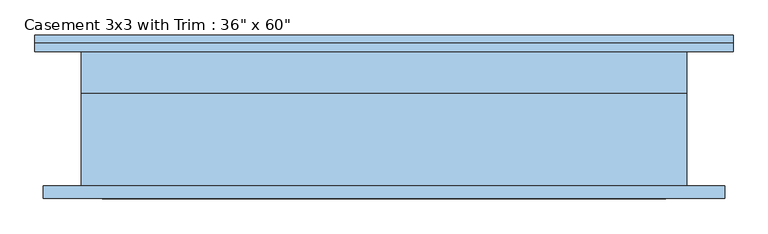
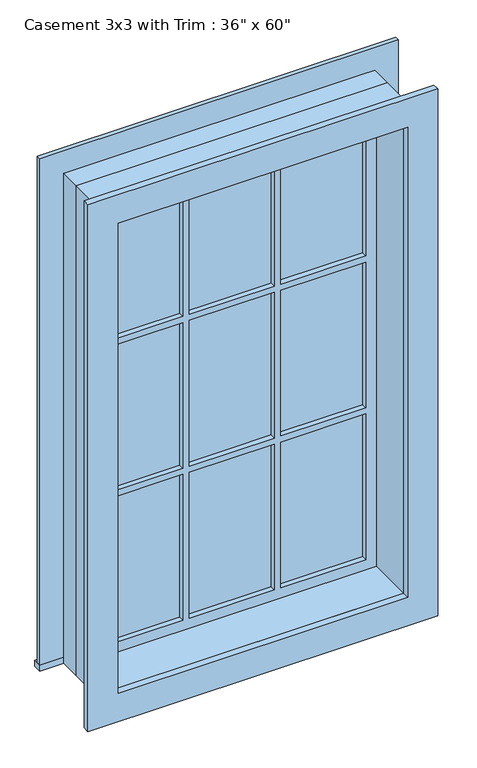
"""IFC4 building model written with IfcOpenShell, lengths in millimetres: window geometry."""

from ifc_helpers import new_model, si_unit, frame, origin, place, context, project, spatial, polyline, outline, extrude, source, transform, mapped, element, save


def window_58e1470a(model_context):
    return source(origin(), model_context, "Body", "SweptSolid", [
        extrude(outline(polyline([(-527.05, 127.0), (527.05, 127.0), (527.05, 101.6), (-527.05, 101.6), (-527.05, 127.0)])), frame((0.0, 0.0, 609.6), z_axis=(0.0, 0.0, 1.0), x_axis=(1.0, 0.0, 0.0)), (0.0, 0.0, 1.0), 19.05),
        extrude(outline(polyline([(2114.55, -438.15), (2114.55, 438.15), (628.65, 438.15), (628.65, 527.05), (2203.45, 527.05), (2203.45, -527.05), (628.65, -527.05), (628.65, -438.15), (2114.55, -438.15)])), frame((0.0, 101.6, 0.0), z_axis=(0.0, 1.0, 0.0), x_axis=(0.0, 0.0, 1.0)), (0.0, 0.0, 1.0), 12.7),
        extrude(outline(polyline([(143.9333333, 66.675), (393.7, 66.675), (393.7, 53.975), (143.9333333, 53.975), (143.9333333, 66.675)])), frame((0.0, 0.0, 1617.1333333), z_axis=(0.0, 0.0, 1.0), x_axis=(1.0, 0.0, 0.0)), (0.0, 0.0, 1.0), 452.9666667),
        extrude(outline(polyline([(-124.8833333, 66.675), (124.8833333, 66.675), (124.8833333, 53.975), (-124.8833333, 53.975), (-124.8833333, 66.675)])), frame((0.0, 0.0, 1617.1333333), z_axis=(0.0, 0.0, 1.0), x_axis=(1.0, 0.0, 0.0)), (0.0, 0.0, 1.0), 452.9666667),
        extrude(outline(polyline([(-393.7, 66.675), (-143.9333333, 66.675), (-143.9333333, 53.975), (-393.7, 53.975), (-393.7, 66.675)])), frame((0.0, 0.0, 1617.1333333), z_axis=(0.0, 0.0, 1.0), x_axis=(1.0, 0.0, 0.0)), (0.0, 0.0, 1.0), 452.9666667),
        extrude(outline(polyline([(-393.7, 66.675), (-143.9333333, 66.675), (-143.9333333, 53.975), (-393.7, 53.975), (-393.7, 66.675)])), frame((0.0, 0.0, 1145.1166667), z_axis=(0.0, 0.0, 1.0), x_axis=(1.0, 0.0, 0.0)), (0.0, 0.0, 1.0), 452.9666667),
        extrude(outline(polyline([(-124.8833333, 66.675), (124.8833333, 66.675), (124.8833333, 53.975), (-124.8833333, 53.975), (-124.8833333, 66.675)])), frame((0.0, 0.0, 1145.1166667), z_axis=(0.0, 0.0, 1.0), x_axis=(1.0, 0.0, 0.0)), (0.0, 0.0, 1.0), 452.9666667),
        extrude(outline(polyline([(143.9333333, 66.675), (393.7, 66.675), (393.7, 53.975), (143.9333333, 53.975), (143.9333333, 66.675)])), frame((0.0, 0.0, 1145.1166667), z_axis=(0.0, 0.0, 1.0), x_axis=(1.0, 0.0, 0.0)), (0.0, 0.0, 1.0), 452.9666667),
        extrude(outline(polyline([(143.9333333, 66.675), (393.7, 66.675), (393.7, 53.975), (143.9333333, 53.975), (143.9333333, 66.675)])), frame((0.0, 0.0, 673.1), z_axis=(0.0, 0.0, 1.0), x_axis=(1.0, 0.0, 0.0)), (0.0, 0.0, 1.0), 452.9666667),
        extrude(outline(polyline([(-124.8833333, 66.675), (124.8833333, 66.675), (124.8833333, 53.975), (-124.8833333, 53.975), (-124.8833333, 66.675)])), frame((0.0, 0.0, 673.1), z_axis=(0.0, 0.0, 1.0), x_axis=(1.0, 0.0, 0.0)), (0.0, 0.0, 1.0), 452.9666667),
        extrude(outline(polyline([(-393.7, 66.675), (-143.9333333, 66.675), (-143.9333333, 53.975), (-393.7, 53.975), (-393.7, 66.675)])), frame((0.0, 0.0, 673.1), z_axis=(0.0, 0.0, 1.0), x_axis=(1.0, 0.0, 0.0)), (0.0, 0.0, 1.0), 452.9666667),
        extrude(outline(polyline([(2190.75, 514.35), (2190.75, -514.35), (552.45, -514.35), (552.45, 514.35), (2190.75, 514.35)]), holes=[polyline([(2101.85, 425.45), (641.35, 425.45), (641.35, -425.45), (2101.85, -425.45), (2101.85, 425.45)])]), frame((0.0, -120.65, 0.0), z_axis=(0.0, 1.0, 0.0), x_axis=(0.0, 0.0, 1.0)), (0.0, 0.0, 1.0), 19.05),
        extrude(outline(polyline([(2114.55, -438.15), (628.65, -438.15), (628.65, 438.15), (2114.55, 438.15), (2114.55, -438.15)]), holes=[polyline([(2070.1, -143.9333333), (1617.1333333, -143.9333333), (1617.1333333, -393.7), (2070.1, -393.7), (2070.1, -143.9333333)]), polyline([(1598.0833333, -143.9333333), (1145.1166667, -143.9333333), (1145.1166667, -393.7), (1598.0833333, -393.7), (1598.0833333, -143.9333333)]), polyline([(1126.0666667, -143.9333333), (673.1, -143.9333333), (673.1, -393.7), (1126.0666667, -393.7), (1126.0666667, -143.9333333)]), polyline([(2070.1, 124.8833333), (1617.1333333, 124.8833333), (1617.1333333, -124.8833333), (2070.1, -124.8833333), (2070.1, 124.8833333)]), polyline([(1598.0833333, 124.8833333), (1145.1166667, 124.8833333), (1145.1166667, -124.8833333), (1598.0833333, -124.8833333), (1598.0833333, 124.8833333)]), polyline([(1126.0666667, 124.8833333), (673.1, 124.8833333), (673.1, -124.8833333), (1126.0666667, -124.8833333), (1126.0666667, 124.8833333)]), polyline([(2070.1, 393.7), (1617.1333333, 393.7), (1617.1333333, 143.9333333), (2070.1, 143.9333333), (2070.1, 393.7)]), polyline([(1598.0833333, 393.7), (1145.1166667, 393.7), (1145.1166667, 143.9333333), (1598.0833333, 143.9333333), (1598.0833333, 393.7)]), polyline([(1126.0666667, 393.7), (673.1, 393.7), (673.1, 143.9333333), (1126.0666667, 143.9333333), (1126.0666667, 393.7)])]), frame((0.0, 38.1, 0.0), z_axis=(0.0, 1.0, 0.0), x_axis=(0.0, 0.0, 1.0)), (0.0, 0.0, 1.0), 44.45),
        extrude(outline(polyline([(2133.6, -457.2), (609.6, -457.2), (609.6, 457.2), (2133.6, 457.2), (2133.6, -457.2)]), holes=[polyline([(2101.85, -425.45), (2101.85, 425.45), (641.35, 425.45), (641.35, -425.45), (2101.85, -425.45)])]), frame((0.0, -101.6, 0.0), z_axis=(0.0, 1.0, 0.0), x_axis=(0.0, 0.0, 1.0)), (0.0, 0.0, 1.0), 139.7),
        extrude(outline(polyline([(2133.6, 457.2), (2133.6, -457.2), (609.6, -457.2), (609.6, 457.2), (2133.6, 457.2)]), holes=[polyline([(2114.55, 438.15), (628.65, 438.15), (628.65, -438.15), (2114.55, -438.15), (2114.55, 438.15)])]), frame((0.0, 38.1, 0.0), z_axis=(0.0, 1.0, 0.0), x_axis=(0.0, 0.0, 1.0)), (0.0, 0.0, 1.0), 63.5),
    ])


if __name__ == "__main__":
    model = new_model("IFC4")
    model_context = context("Model", 3, world=origin())
    ifc_project = project(units=[si_unit("LENGTHUNIT", "METRE", prefix="MILLI")], contexts=[model_context])
    site = spatial("IfcSite", under=ifc_project)
    building = spatial("IfcBuilding", under=site)
    placement = place(None, origin())
    window_shape = window_58e1470a(model_context)
    element("IfcWindow", 1, ObjectType="Casement 3x3 with Trim : 36\" x 60\"", at=placement, inside=building, context=model_context, shape_type="MappedRepresentation", body=[
        mapped(window_shape, transform((0.0, 0.0, 0.0), x_axis=(1.0, 0.0, 0.0), y_axis=(0.0, 1.0, 0.0), z_axis=(0.0, 0.0, 1.0))),
    ])
    save(model, "model.ifc")

# Revit data of these elements
# Type "Casement 3x3 with Trim : 36\" x 60\""
#   Type Mark = "14"
#   Construction Type Id = "GSP4R"
#   Assembly Code = "B2020100"
#   Analytic Construction = "1/8 in Pilkington single glazing"
#   Visual Light Transmittance = 0.9
#   Solar Heat Gain Coefficient = 0.78
#   Heat Transfer Coefficient (U) = 0.6496 BTU/(h·ft²·°F)
#   Height = 5' - 0"
#   Default Sill Height = 2' - 0"
#   Trim Projection - Ext. = 0' - 0 1/2"
#   Trim Projection - Int. = 0' - 0 3/4"
#   Trim Width - Exterior = 0' - 3 1/2"
#   Trim Width - Interior = 0' - 3 1/2"
#   Width = 3' - 0"
#   Window Inset = 0' - 0 3/4"
#   Define Thermal Properties by = 1
#   Glass Pane Material = Glass
#   Sash Material = Sash
#   Trim Exterior Material = Trim
#   Trim Interior Material = Trim
#   Wall Closure = (empty or 0)
# Element 1 (IfcWindow, "Casement 3x3 with Trim : 36\" x 60\"")
#   Materials on its faces: "Sash", "Glass", "Trim"
# Materials
#   "Glass": class "Glass", colour RGB 0 128 192, transparency 0.75, Description = "Soda Lime Glass", Cost = 0
#   "Sash": class "Wood", colour RGB 224 178 126, transparency 0
#   "Trim": class "Wood", colour RGB 224 178 126, transparency 0
